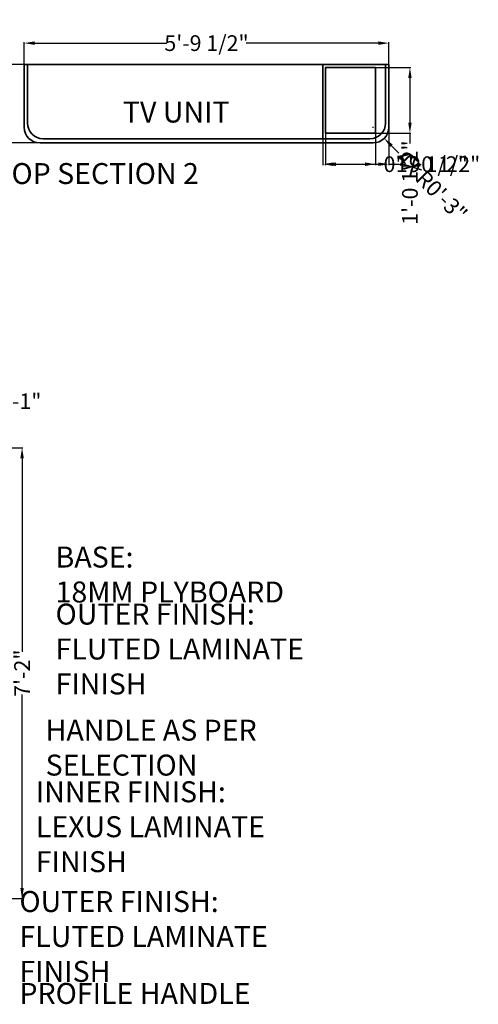
# Model space of a CAD drawing. Units: inches. Extents: x 5 to 197, y 46 to 234.
# Tile 2 of 2: x 109 to 197, y 46 to 234. Entities that reach past the tile are written whole.
import ezdxf

# ---------------------------------------------------------------- set-up
doc = ezdxf.new("R2010")
doc.units = ezdxf.units.IN
doc.header["$MEASUREMENT"] = 0
for name, color, linetype, lineweight in [('A-ANNO-DIMS', 2, 'Continuous', 18), ('A-ANNO-TEXT', 3, 'Continuous', 18), ('A-SECT', 7, 'Continuous', 35)]:
    doc.layers.add(name, color=color, linetype=linetype, lineweight=lineweight)
doc.styles.get("Standard").update_dxf_attribs({"font": 'arial.ttf'})
doc.dimstyles.get("Standard").update_dxf_attribs({"dimtxt": 3, "dimasz": 2, "dimexe": 0.18, "dimexo": 0.0625, "dimgap": 0.09, "dimtad": 0, "dimdec": 0, "dimzin": 0, "dimdsep": 46, "dimlunit": 4, "dimtxsty": 'Standard', "dimcen": 0.09, "dimadec": 0, "dimazin": 0, "dimtfac": 1, "dimtdec": 0, "dimtofl": 0, "dimtmove": 0, "dimatfit": 3, "dimfxl": 1, "dimtolj": 1, "dimtzin": 0, "dimarcsym": 1})

# ---------------------------------------------------------------- blocks, each defined once
blk = doc.blocks.new('*D22')
at = {"layer": 'A-ANNO-DIMS', "color": 0, "lineweight": -2, "transparency": 16777216}
for p, q in [((100.64, 152.66), (109.65, 152.66)), ((109.47, 150.66), (109.47, 113.72)), ((109.47, 68.66), (109.47, 105.59)), ((100.64, 66.66), (109.65, 66.66))]:
    blk.add_line(p, q, dxfattribs=at)
at = {"layer": 'A-ANNO-DIMS', "color": 0, "transparency": 16777216}
for points in [[(109.14, 150.66), (109.81, 150.66), (109.47, 152.66)], [(109.14, 68.66), (109.81, 68.66), (109.47, 66.66)]]:
    blk.add_solid(points, dxfattribs=at)
at = {"layer": 'Defpoints', "color": 0, "transparency": 16777216}
for p in [(100.57, 152.66), (109.47, 152.66), (100.57, 66.66)]:
    blk.add_point(p, dxfattribs=at)
at = {"layer": 'A-ANNO-DIMS', "color": 0, "transparency": 16777216, "insert": (109.47, 109.66), "char_height": 3, "attachment_point": 5, "rotation": 90}
blk.add_mtext('\\A1;7\'-2"', dxfattribs=at)
blk = doc.blocks.new('*D28')
at = {"layer": 'A-ANNO-DIMS', "color": 0, "lineweight": -2, "transparency": 16777216}
for p, q in [((99.57, 152.72), (99.57, 161.74)), ((100.57, 152.72), (100.57, 161.74)), ((97.57, 161.56), (95.57, 161.56)), ((102.57, 161.56), (104.57, 161.56))]:
    blk.add_line(p, q, dxfattribs=at)
at = {"layer": 'A-ANNO-DIMS', "color": 0, "transparency": 16777216}
for points in [[(97.57, 161.89), (97.57, 161.22), (99.57, 161.56)], [(102.57, 161.89), (102.57, 161.22), (100.57, 161.56)]]:
    blk.add_solid(points, dxfattribs=at)
at = {"layer": 'Defpoints', "color": 0, "transparency": 16777216}
for p in [(100.57, 161.56), (99.57, 152.66), (100.57, 152.66)]:
    blk.add_point(p, dxfattribs=at)
at = {"layer": 'A-ANNO-DIMS', "color": 0, "transparency": 16777216, "insert": (108.65, 161.56), "char_height": 3, "attachment_point": 5}
blk.add_mtext('\\A1;0\'-1"', dxfattribs=at)
blk = doc.blocks.new('*D30')
at = {"layer": 'A-ANNO-DIMS', "color": 0, "lineweight": -2, "transparency": 16777216}
for p, q in [((167.41, 212.65), (167.41, 206.61)), ((176.99, 212.65), (176.99, 206.61)), ((169.41, 206.79), (174.99, 206.79)), ((176.99, 206.79), (178.99, 206.79))]:
    blk.add_line(p, q, dxfattribs=at)
at = {"layer": 'A-ANNO-DIMS', "color": 0, "transparency": 16777216}
for points in [[(169.41, 207.12), (169.41, 206.45), (167.41, 206.79)], [(174.99, 207.12), (174.99, 206.45), (176.99, 206.79)]]:
    blk.add_solid(points, dxfattribs=at)
at = {"layer": 'Defpoints', "color": 0, "transparency": 16777216}
for p in [(167.41, 212.71), (176.99, 212.71), (176.99, 206.79)]:
    blk.add_point(p, dxfattribs=at)
at = {"layer": 'A-ANNO-DIMS', "color": 0, "transparency": 16777216, "insert": (186.56, 206.79), "char_height": 3, "attachment_point": 5}
blk.add_mtext('\\A1;0\'-9 1/2"', dxfattribs=at)
blk = doc.blocks.new('*D31')
at = {"layer": 'A-ANNO-DIMS', "color": 0, "lineweight": -2, "transparency": 16777216}
for p, q in [((179.5, 213.78), (179.5, 206.61)), ((166.9, 211.58), (166.9, 206.61)), ((168.9, 206.79), (177.5, 206.79)), ((179.5, 206.79), (181.5, 206.79))]:
    blk.add_line(p, q, dxfattribs=at)
at = {"layer": 'A-ANNO-DIMS', "color": 0, "transparency": 16777216}
for points in [[(168.9, 207.12), (168.9, 206.45), (166.9, 206.79)], [(177.5, 207.12), (177.5, 206.45), (179.5, 206.79)]]:
    blk.add_solid(points, dxfattribs=at)
at = {"layer": 'Defpoints', "color": 0, "transparency": 16777216}
for p in [(179.5, 213.84), (166.9, 211.64), (179.5, 206.79)]:
    blk.add_point(p, dxfattribs=at)
at = {"layer": 'A-ANNO-DIMS', "color": 0, "transparency": 16777216, "insert": (188.93, 206.79), "char_height": 3, "attachment_point": 5}
blk.add_mtext('\\A1;1\'-0 1/2"', dxfattribs=at)
blk = doc.blocks.new('*D32')
at = {"layer": 'A-ANNO-DIMS', "color": 0, "lineweight": -2, "transparency": 16777216}
for p, q in [((109.9, 225.9), (109.9, 230.07)), ((111.9, 229.89), (137.13, 229.89)), ((177.5, 229.89), (152.27, 229.89)), ((179.5, 225.9), (179.5, 230.07))]:
    blk.add_line(p, q, dxfattribs=at)
at = {"layer": 'A-ANNO-DIMS', "color": 0, "transparency": 16777216}
for points in [[(111.9, 230.22), (111.9, 229.55), (109.9, 229.89)], [(177.5, 230.22), (177.5, 229.55), (179.5, 229.89)]]:
    blk.add_solid(points, dxfattribs=at)
at = {"layer": 'Defpoints', "color": 0, "transparency": 16777216}
for p in [(179.5, 229.89), (109.9, 225.84), (179.5, 225.84)]:
    blk.add_point(p, dxfattribs=at)
at = {"layer": 'A-ANNO-DIMS', "color": 0, "transparency": 16777216, "insert": (144.7, 229.89), "char_height": 3, "attachment_point": 5}
blk.add_mtext('\\A1;5\'-9 1/2"', dxfattribs=at)
blk = doc.blocks.new('*D33')
at = {"layer": 'A-ANNO-DIMS', "color": 0, "lineweight": -2, "transparency": 16777216}
for p, q in [((109.84, 225.84), (105.67, 225.84)), ((105.85, 223.84), (105.85, 222.27)), ((105.85, 212.84), (105.85, 214.4)), ((112.84, 210.84), (105.67, 210.84))]:
    blk.add_line(p, q, dxfattribs=at)
at = {"layer": 'A-ANNO-DIMS', "color": 0, "transparency": 16777216}
for points in [[(105.52, 223.84), (106.18, 223.84), (105.85, 225.84)], [(105.52, 212.84), (106.18, 212.84), (105.85, 210.84)]]:
    blk.add_solid(points, dxfattribs=at)
at = {"layer": 'Defpoints', "color": 0, "transparency": 16777216}
for p in [(109.9, 225.84), (105.85, 210.84), (112.9, 210.84)]:
    blk.add_point(p, dxfattribs=at)
at = {"layer": 'A-ANNO-DIMS', "color": 0, "transparency": 16777216, "insert": (105.85, 218.34), "char_height": 3, "attachment_point": 5, "rotation": 90}
blk.add_mtext('\\A1;1\'-3"', dxfattribs=at)
blk = doc.blocks.new('*D34')
at = {"layer": 'A-ANNO-DIMS', "color": 0, "lineweight": -2, "transparency": 16777216}
for p, q in [((177.05, 225.21), (183.73, 225.21)), ((183.55, 223.21), (183.55, 214.71)), ((177.05, 212.71), (183.73, 212.71)), ((183.55, 212.71), (183.55, 210.71))]:
    blk.add_line(p, q, dxfattribs=at)
at = {"layer": 'A-ANNO-DIMS', "color": 0, "transparency": 16777216}
for points in [[(183.22, 223.21), (183.88, 223.21), (183.55, 225.21)], [(183.22, 214.71), (183.88, 214.71), (183.55, 212.71)]]:
    blk.add_solid(points, dxfattribs=at)
at = {"layer": 'Defpoints', "color": 0, "transparency": 16777216}
for p in [(176.99, 225.21), (176.99, 212.71), (183.55, 212.71)]:
    blk.add_point(p, dxfattribs=at)
at = {"layer": 'A-ANNO-DIMS', "color": 0, "transparency": 16777216, "insert": (183.55, 203.28), "char_height": 3, "attachment_point": 5, "rotation": 90}
blk.add_mtext('\\A1;1\'-0 1/2"', dxfattribs=at)
blk = doc.blocks.new('*D37')
at = {"layer": 'A-ANNO-DIMS', "color": 0, "lineweight": -2, "transparency": 16777216}
for p, q in [((176.41, 213.84), (176.59, 213.84)), ((176.5, 213.75), (176.5, 213.93)), ((181.45, 208.89), (180.04, 210.3))]:
    blk.add_line(p, q, dxfattribs=at)
at = {"layer": 'A-ANNO-DIMS', "color": 0, "transparency": 16777216}
blk.add_solid([(180.27, 210.54), (179.8, 210.07), (178.62, 211.72)], dxfattribs=at)
at = {"layer": 'Defpoints', "color": 0, "transparency": 16777216}
for p in [(176.5, 213.84), (178.62, 211.72)]:
    blk.add_point(p, dxfattribs=at)
at = {"layer": 'A-ANNO-DIMS', "color": 0, "transparency": 16777216, "insert": (187.67, 202.67), "char_height": 3, "attachment_point": 5, "rotation": 314.9952}
blk.add_mtext('\\A1;4X R0\'-3"', dxfattribs=at)

msp = doc.modelspace()

# ---------------------------------------------------------------- linework, layer by layer
at = {"layer": 'A-SECT'}
for p, q in [((179.5, 225.84), (109.9, 225.84)), ((109.9, 225.84), (109.9, 213.84)), ((110.5, 225.84), (110.5, 214.64)), ((166.9, 225.84), (166.9, 211.64)), ((178.9, 225.84), (178.9, 214.64)), ((179.5, 225.84), (179.5, 213.84)), ((112.9, 210.84), (176.5, 210.84)), ((113.5, 211.64), (175.9, 211.64))]:
    msp.add_line(p, q, dxfattribs=at)
msp.add_lwpolyline([(176.99, 212.71), (167.41, 212.71), (167.41, 225.21), (176.99, 225.21)], close=True, dxfattribs=at)
for centre, start, end in [((113.5, 214.64), 180, 270), ((175.9, 214.64), 270, 0), ((112.9, 213.84), 180, 270), ((176.5, 213.84), 270, 0)]:
    msp.add_arc(centre, 3, start, end, dxfattribs=at)

# ---------------------------------------------------------------- texts
at = {"layer": 'A-ANNO-TEXT', "char_height": 4, "attachment_point": 1}
for s, width, insert in [('TV UNIT', 71.1037, (128.73, 218.74)), ('TOP SECTION 2', 72.0117, (104.18, 207)), ('BASE:\\P18MM PLYBOARD', 91.3345, (115.87, 133.82)), ('OUTER FINISH:\\PFLUTED LAMINATE \\PFINISH', 92.2198, (115.87, 122.94)), ('HANDLE AS PER  \\PSELECTION', 79.123, (113.97, 100.79)), ('INNER FINISH:\\PLEXUS LAMINATE\\PFINISH', 98.6635, (112.1, 89.03)), ('OUTER FINISH:\\PFLUTED LAMINATE \\PFINISH', 92.2198, (108.97, 68.09)), ('PROFILE HANDLE', 108.1629, (108.97, 50.55))]:
    msp.add_mtext_dynamic_manual_height_columns(s, width=width, gutter_width=20, heights=[0], dxfattribs=dict(at, insert=insert))

# ---------------------------------------------------------------- dimensions: what is measured, and where the dimension line sits
at = {"layer": 'A-ANNO-DIMS'}
for base, p1, p2, picture, middle in [((179.5, 229.89), (109.9, 225.84), (179.5, 225.84), '*D32', (144.7, 229.89)), ((179.5, 206.79), (166.9, 211.64), (179.5, 213.84), '*D31', (188.93, 206.79)), ((176.99, 206.79), (167.41, 212.71), (176.99, 212.71), '*D30', (186.56, 206.79)), ((100.57, 161.56), (99.57, 152.66), (100.57, 152.66), '*D28', (108.65, 161.56))]:
    dim = msp.add_linear_dim(base=base, p1=p1, p2=p2, dimstyle='Standard', override={"dimdec": 1, "dimlfac": 1, "dimrnd": 0, "dimzin": 1, "dimdsep": 46, "dimlunit": 4, "dimfrac": 2}, dxfattribs=at)
    dim.commit()
    dim.dimension.update_dxf_attribs({"geometry": picture, "text_midpoint": middle})
for base, p1, p2, picture, middle in [((105.85, 210.84), (109.9, 225.84), (112.9, 210.84), '*D33', (105.85, 218.34)), ((183.55, 212.71), (176.99, 225.21), (176.99, 212.71), '*D34', (183.55, 203.28)), ((109.47, 152.66), (100.57, 66.66), (100.57, 152.66), '*D22', (109.47, 109.66))]:
    dim = msp.add_linear_dim(base=base, p1=p1, p2=p2, angle=90, dimstyle='Standard', override={"dimdec": 1, "dimlfac": 1, "dimrnd": 0, "dimzin": 1, "dimdsep": 46, "dimlunit": 4, "dimfrac": 2}, dxfattribs=at)
    dim.commit()
    dim.dimension.update_dxf_attribs({"geometry": picture, "text_midpoint": middle})
dim = msp.add_radius_dim(center=(176.5, 213.84), mpoint=(178.62, 211.72), text='4X <>', dimstyle='Standard', override={"dimdec": 1, "dimlfac": 1, "dimrnd": 0, "dimzin": 1, "dimdsep": 46, "dimlunit": 4, "dimfrac": 2}, dxfattribs=at)
dim.commit()
dim.dimension.update_dxf_attribs({"geometry": '*D37', "text_midpoint": (187.67, 202.67)})

doc.saveas('drawing.dxf')
